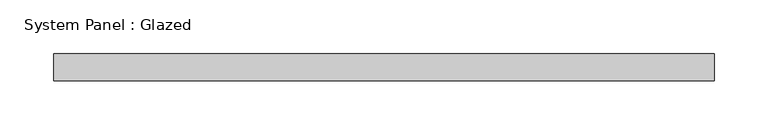
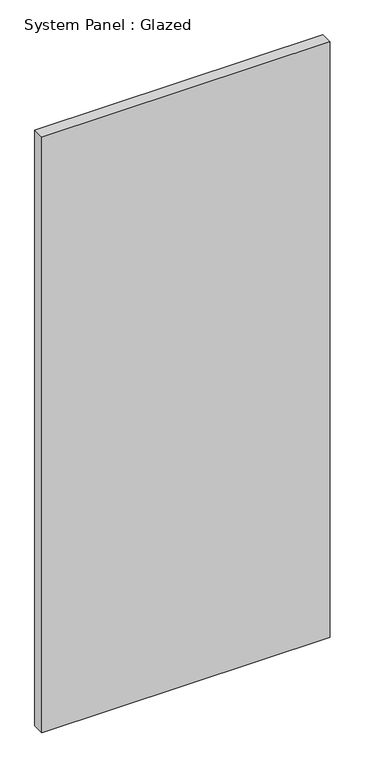
"""IFC4 building model written with IfcOpenShell, lengths in millimetres: plate geometry, System Panel : Glazed."""

from ifc_helpers import new_model, si_unit, origin, origin_with_axes, place, context, project, spatial, polyline, outline, extrude, source, transform, mapped, element, save


def system_panel_glazed_bfa5483a(model_context):
    return source(origin(), model_context, "Body", "SweptSolid", [
        extrude(outline(polyline([(307.975, 19.05), (-307.975, 19.05), (-307.975, 44.45), (307.975, 44.45), (307.975, 19.05)])), origin_with_axes(), (0.0, 0.0, 1.0), 1345.6043316),
    ])


if __name__ == "__main__":
    model = new_model("IFC4")
    model_context = context("Model", 3, world=origin())
    ifc_project = project(units=[si_unit("LENGTHUNIT", "METRE", prefix="MILLI")], contexts=[model_context])
    site = spatial("IfcSite", under=ifc_project)
    building = spatial("IfcBuilding", under=site)
    placement = place(None, origin())
    system_panel_glazed_shape = system_panel_glazed_bfa5483a(model_context)
    element("IfcPlate", 1, ObjectType="System Panel : Glazed", at=placement, inside=building, context=model_context, shape_type="MappedRepresentation", body=[
        mapped(system_panel_glazed_shape, transform((0.0, 0.0, 0.0), x_axis=(1.0, 0.0, 0.0), y_axis=(0.0, 1.0, 0.0), z_axis=(0.0, 0.0, 1.0))),
    ])
    save(model, "model.ifc")

# Revit data of these elements
# Type "System Panel : Glazed"
#   Construction Type Id = "GSP4R"
#   Analytic Construction = "1/8 in Pilkington single glazing"
#   Visual Light Transmittance = 0.9
#   Solar Heat Gain Coefficient = 0.86
#   Heat Transfer Coefficient (U) = 1.18115 BTU/(h·ft²·°F)
#   Define Thermal Properties by = 1
# Element 1 (IfcPlate, "System Panel : Glazed")
#   Materials on its faces: "Glass"
# Materials
#   "Glass": class "Glass", colour RGB 0 128 192, transparency 0.75, Description = "Soda Lime Glass", Cost = 0
